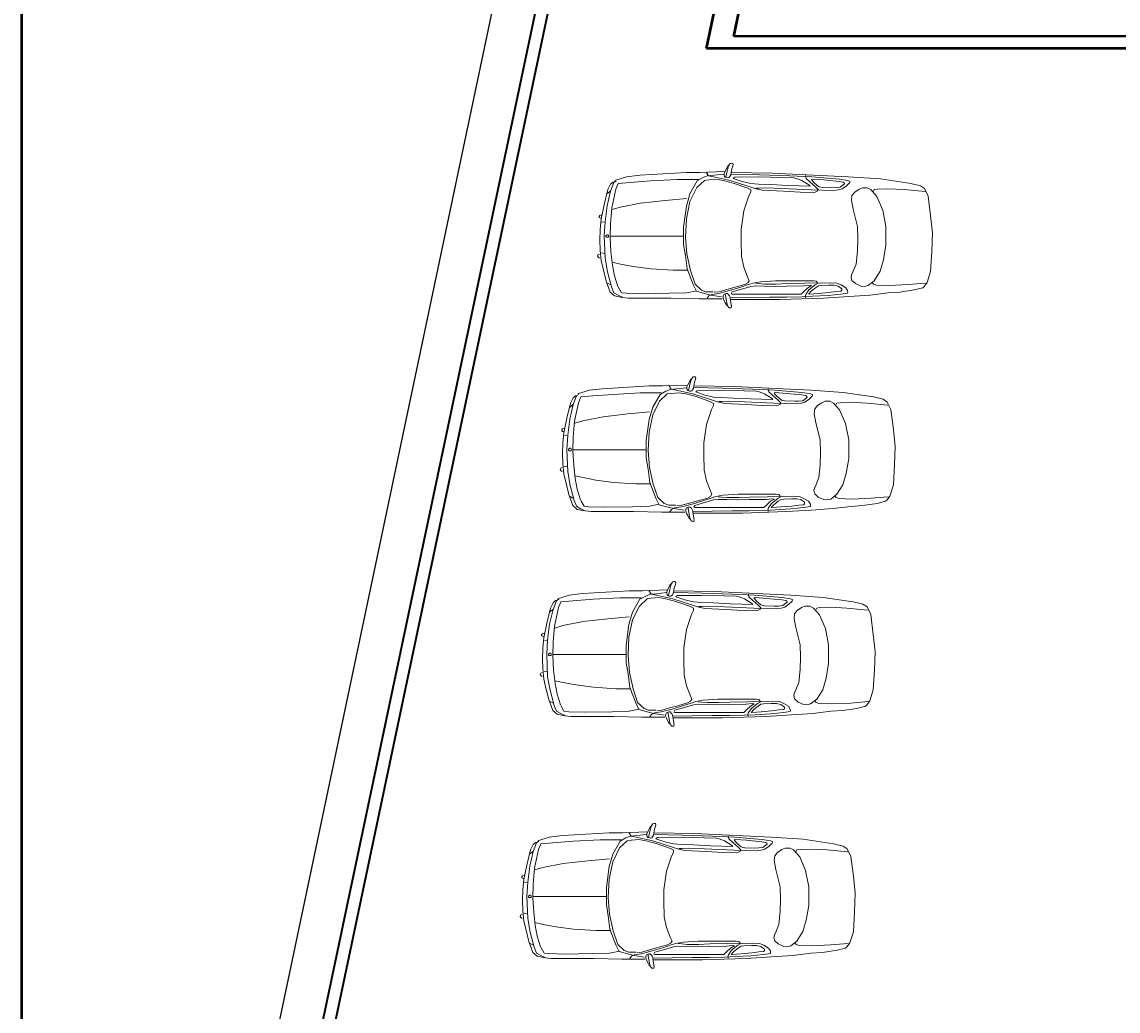
# Model space of a CAD drawing. Units: millimetres. Extents: x 2134 to 3363, y 1052 to 3233.
# Tile 2 of 11: x 2134 to 2539, y 1417 to 1782. Entities that reach past the tile are written whole.
import ezdxf

# ---------------------------------------------------------------- set-up
doc = ezdxf.new("R2010")
doc.units = ezdxf.units.MM
for name, color, linetype, lineweight in [('A-ANNO-DIMS', 2, 'Continuous', 18), ('A-ANNO-TTLB', 7, 'Continuous', 50), ('A-SITE-PRKG', 8, 'Continuous', 13), ('A-WALL', 7, 'Continuous', 50), ('C-PROP', 6, 'Continuous', 35)]:
    doc.layers.add(name, color=color, linetype=linetype, lineweight=lineweight)
doc.styles.get("Standard").update_dxf_attribs({"font": 'arial.ttf'})
doc.dimstyles.new('ISO-25', dxfattribs={"dimtxt": 2.5, "dimasz": 2.5, "dimexe": 1.25, "dimexo": 0.625, "dimtad": 1, "dimtxsty": 'Standard', "dimcen": 2.5, "dimadec": 0, "dimazin": 0, "dimtfac": 1, "dimtmove": 0, "dimatfit": 3, "dimfxl": 1, "dimarcsym": 0})

# ---------------------------------------------------------------- blocks, each defined once
blk = doc.blocks.new('A$C52303110')
for p, q in [((-0.168, 1.141), (-0.185, 1.111)), ((-0.162, 1.148), (-0.168, 1.141)), ((-0.142, 1.15), (-0.162, 1.148)), ((-0.13, 1.15), (-0.142, 1.15)), ((-0.123, 1.145), (-0.13, 1.15)), ((-0.117, 1.134), (-0.123, 1.145)), ((-0.123, 1.109), (-0.117, 1.134)), ((-1.693, 0.951), (-1.496, 0.973)), ((-1.496, 0.973), (-0.807, 1.016)), ((-0.807, 1.016), (-0.61, 1.016)), ((-0.61, 1.016), (-0.252, 1.027)), ((-0.517, 1.02), (-0.48, 0.966)), ((-0.256, 0.988), (-0.404, 0.972)), ((-0.237, 1.032), (-0.251, 1.001)), ((-0.251, 1.001), (-0.25, 0.98)), ((-0.25, 0.98), (-0.245, 0.957)), ((-0.198, 1.106), (-0.237, 1.032)), ((-0.206, 1.035), (-0.226, 0.944)), ((-0.185, 1.111), (-0.206, 1.035)), ((-0.184, 1.117), (-0.198, 1.106)), ((-0.167, 0.957), (-0.154, 0.98)), ((-0.154, 0.98), (-0.148, 1.013)), ((-0.148, 1.013), (-0.144, 1.04)), ((-0.145, 0.991), (0.272, 0.981)), ((-0.144, 1.04), (-0.137, 1.07)), ((-0.144, 1.016), (0.455, 1.005)), ((-0.137, 1.07), (-0.123, 1.109)), ((0.272, 0.981), (0.721, 0.966)), ((0.455, 1.005), (1.583, 0.951)), ((-1.969, 0.76), (-1.928, 0.839)), ((-1.928, 0.839), (-1.887, 0.875)), ((-1.928, 0.738), (-1.881, 0.868)), ((-1.881, 0.868), (-1.846, 0.889)), ((-1.863, 0.896), (-1.693, 0.951)), ((-1.852, 0.767), (-1.816, 0.853)), ((-1.816, 0.853), (-1.64, 0.868)), ((-1.64, 0.868), (-1.339, 0.889)), ((-1.339, 0.889), (-0.939, 0.911)), ((-0.939, 0.911), (-0.698, 0.911)), ((-0.647, 0.889), (-0.755, 0.7)), ((-0.698, 0.911), (-0.627, 0.911)), ((-0.539, 0.897), (-0.654, 0.79)), ((-0.56, 0.938), (-0.647, 0.889)), ((-0.499, 0.963), (-0.56, 0.938)), ((-0.479, 0.905), (-0.539, 0.897)), ((-0.404, 0.972), (-0.499, 0.963)), ((-0.48, 0.966), (-0.383, 0.946)), ((-0.371, 0.914), (-0.479, 0.905)), ((-0.383, 0.946), (-0.161, 0.897)), ((-0.263, 0.897), (-0.371, 0.914)), ((-0.115, 0.856), (-0.263, 0.897)), ((-0.245, 0.957), (-0.234, 0.947)), ((-0.234, 0.947), (-0.213, 0.938)), ((-0.213, 0.938), (-0.192, 0.936)), ((-0.192, 0.936), (-0.179, 0.942)), ((-0.179, 0.942), (-0.167, 0.957)), ((-0.161, 0.897), (0.098, 0.813)), ((-0.119, 0.926), (-0.109, 0.937)), ((0.017, 0.88), (-0.119, 0.926)), ((0.101, 0.782), (-0.115, 0.856)), ((-0.109, 0.937), (-0.091, 0.944)), ((-0.091, 0.944), (0.26, 0.948)), ((0.143, 0.85), (0.017, 0.88)), ((0.098, 0.813), (0.203, 0.778)), ((0.257, 0.843), (0.143, 0.85)), ((0.441, 0.835), (0.257, 0.843)), ((0.26, 0.948), (0.598, 0.941)), ((0.69, 0.824), (0.441, 0.835)), ((0.598, 0.941), (0.777, 0.937)), ((1.022, 0.813), (0.69, 0.824)), ((0.721, 0.966), (1.045, 0.951)), ((0.777, 0.937), (0.817, 0.926)), ((0.817, 0.926), (0.897, 0.896)), ((0.897, 0.896), (1.001, 0.832)), ((0.956, 0.951), (0.952, 0.971)), ((0.96, 0.926), (0.956, 0.951)), ((1.016, 0.877), (0.96, 0.926)), ((1.001, 0.832), (1.022, 0.813)), ((1.105, 0.798), (1.016, 0.877)), ((1.038, 0.912), (1.054, 0.916)), ((1.043, 0.899), (1.038, 0.912)), ((1.082, 0.858), (1.043, 0.899)), ((1.045, 0.951), (1.453, 0.917)), ((1.054, 0.916), (1.221, 0.903)), ((1.141, 0.807), (1.082, 0.858)), ((1.221, 0.903), (1.447, 0.882)), ((1.447, 0.882), (1.506, 0.871)), ((1.453, 0.917), (1.579, 0.897)), ((1.508, 0.83), (1.464, 0.796)), ((1.555, 0.818), (1.494, 0.773)), ((1.506, 0.871), (1.524, 0.86)), ((1.527, 0.847), (1.508, 0.83)), ((1.524, 0.86), (1.527, 0.847)), ((1.603, 0.862), (1.555, 0.818)), ((1.579, 0.897), (1.611, 0.882)), ((1.583, 0.951), (2.058, 0.918)), ((1.611, 0.882), (1.603, 0.862)), ((2.058, 0.918), (2.505, 0.852)), ((2.505, 0.852), (2.648, 0.819)), ((2.648, 0.819), (2.711, 0.776)), ((-2.022, 0.537), (-1.969, 0.76)), ((-1.981, 0.523), (-1.928, 0.738)), ((-1.975, 0.702), (-1.934, 0.738)), ((-1.91, 0.494), (-1.852, 0.767)), ((-0.755, 0.7), (-0.809, 0.518)), ((-0.654, 0.79), (-0.755, 0.585)), ((0.04, 0.445), (0.115, 0.667)), ((0.142, 0.757), (0.101, 0.782)), ((0.115, 0.667), (0.142, 0.724)), ((0.142, 0.724), (0.142, 0.757)), ((0.203, 0.778), (0.312, 0.754)), ((0.268, 0.783), (0.22, 0.783)), ((0.361, 0.788), (0.268, 0.783)), ((0.312, 0.754), (0.624, 0.739)), ((0.6, 0.778), (0.361, 0.788)), ((1.037, 0.759), (0.6, 0.778)), ((0.624, 0.739), (0.871, 0.724)), ((0.871, 0.724), (1.077, 0.719)), ((1.364, 0.748), (1.037, 0.759)), ((1.077, 0.719), (1.13, 0.739)), ((1.138, 0.763), (1.105, 0.798)), ((1.13, 0.739), (1.138, 0.763)), ((1.159, 0.801), (1.141, 0.807)), ((1.199, 0.794), (1.159, 0.801)), ((1.338, 0.788), (1.199, 0.794)), ((1.403, 0.79), (1.338, 0.788)), ((1.437, 0.759), (1.364, 0.748)), ((1.464, 0.796), (1.403, 0.79)), ((1.494, 0.773), (1.437, 0.759)), ((1.638, 0.675), (1.632, 0.604)), ((1.678, 0.724), (1.638, 0.675)), ((1.742, 0.767), (1.678, 0.724)), ((1.794, 0.788), (1.742, 0.767)), ((1.863, 0.788), (1.794, 0.788)), ((1.915, 0.76), (1.863, 0.788)), ((2.007, 0.661), (1.915, 0.76)), ((1.955, 0.738), (1.967, 0.76)), ((1.967, 0.76), (2.013, 0.767)), ((2.094, 0.457), (2.007, 0.661)), ((2.013, 0.767), (2.169, 0.774)), ((2.169, 0.774), (2.411, 0.76)), ((2.411, 0.76), (2.717, 0.731)), ((2.711, 0.776), (2.765, 0.666)), ((2.765, 0.666), (2.8, 0.371)), ((-2.069, 0.322), (-2.022, 0.537)), ((-2.01, 0.285), (-1.981, 0.523)), ((-1.928, 0.257), (-1.91, 0.494)), ((-1.904, 0.465), (-1.787, 0.501)), ((-1.787, 0.501), (-1.487, 0.559)), ((-1.487, 0.559), (-1.122, 0.602)), ((-1.122, 0.602), (-0.804, 0.631)), ((-0.809, 0.518), (-0.849, 0.206)), ((-0.755, 0.585), (-0.809, 0.329)), ((1.632, 0.604), (1.655, 0.471)), ((-2.087, 0.379), (-2.099, 0.364)), ((-2.099, 0.364), (-2.099, 0.35)), ((-2.099, 0.35), (-2.087, 0.343)), ((-2.064, 0.386), (-2.087, 0.379)), ((-2.087, 0.343), (-2.069, 0.336)), ((-0.809, 0.329), (-0.823, 0.058)), ((0, 0.173), (0.04, 0.445)), ((1.655, 0.471), (1.718, 0.217)), ((2.14, 0.217), (2.094, 0.457)), ((2.8, 0.371), (2.828, 0.12)), ((-2.087, 0.012), (-2.081, 0.17)), ((-2.081, 0.17), (-2.069, 0.322)), ((-2.057, 0.278), (-2.022, 0.285)), ((-2.022, 0.077), (-2.01, 0.285)), ((-1.934, 0.055), (-1.928, 0.257)), ((-0.849, 0.206), (-0.849, -0.049)), ((0, 0), (0, 0.173)), ((1.718, 0.217), (1.724, 0.033)), ((2.14, -0.058), (2.14, 0.217)), ((-2.081, -0.132), (-2.087, 0.012)), ((-2.01, -0.254), (-2.022, 0.077)), ((-1.981, 0.093), (-1.999, 0.079)), ((-1.999, 0.079), (-1.999, 0.064)), ((-1.999, 0.057), (-1.97, 0.057)), ((-1.963, 0.093), (-1.981, 0.093)), ((-1.97, 0.057), (-1.958, 0.057)), ((-1.958, 0.079), (-1.963, 0.093)), ((-1.958, 0.057), (-1.958, 0.079)), ((-1.922, -0.16), (-1.934, 0.055)), ((-1.926, 0.072), (-0.858, 0.072)), ((-0.823, 0.058), (-0.802, -0.19)), ((0.007, -0.23), (0, 0)), ((1.724, 0.033), (1.718, -0.15)), ((2.828, 0.12), (2.819, -0.153)), ((-2.069, -0.29), (-2.081, -0.132)), ((-1.898, -0.354), (-1.922, -0.16)), ((-0.849, -0.049), (-0.823, -0.214)), ((1.718, -0.15), (1.701, -0.34)), ((2.105, -0.277), (2.14, -0.058)), ((2.819, -0.153), (2.8, -0.448)), ((-2.11, -0.2), (-2.122, -0.221)), ((-2.122, -0.221), (-2.11, -0.236)), ((-2.093, -0.193), (-2.11, -0.2)), ((-2.11, -0.236), (-2.093, -0.25)), ((-2.04, -0.405), (-2.069, -0.29)), ((-2.064, -0.175), (-2.016, -0.182)), ((-1.975, -0.455), (-2.01, -0.254)), ((-1.903, -0.313), (-1.782, -0.341)), ((-0.823, -0.214), (-0.796, -0.412)), ((-0.802, -0.19), (-0.748, -0.436)), ((0.04, -0.387), (0.007, -0.23)), ((2.053, -0.446), (2.105, -0.277)), ((-1.993, -0.592), (-2.04, -0.405)), ((-1.916, -0.678), (-1.975, -0.455)), ((-1.869, -0.512), (-1.898, -0.354)), ((-1.782, -0.341), (-1.593, -0.376)), ((-1.593, -0.376), (-1.335, -0.411)), ((-1.335, -0.411), (-1.002, -0.432)), ((-1.002, -0.432), (-0.784, -0.432)), ((-0.796, -0.412), (-0.708, -0.642)), ((-0.748, -0.436), (-0.681, -0.634)), ((0.094, -0.527), (0.04, -0.387)), ((1.638, -0.481), (1.626, -0.531)), ((1.701, -0.34), (1.643, -0.481)), ((1.967, -0.587), (2.053, -0.446)), ((2.8, -0.448), (2.747, -0.612)), ((-1.934, -0.754), (-1.993, -0.592)), ((-1.975, -0.62), (-1.934, -0.642)), ((-1.822, -0.671), (-1.869, -0.512)), ((-0.708, -0.642), (-0.661, -0.741)), ((-0.681, -0.634), (-0.586, -0.724)), ((-0.088, -0.683), (0.054, -0.642)), ((-0.002, -0.68), (0.109, -0.643)), ((0.054, -0.642), (0.101, -0.617)), ((0.121, -0.585), (0.094, -0.527)), ((0.101, -0.617), (0.121, -0.585)), ((0.109, -0.643), (0.178, -0.62)), ((0.178, -0.62), (0.288, -0.601)), ((0.266, -0.629), (0.212, -0.624)), ((0.346, -0.634), (0.266, -0.629)), ((0.288, -0.601), (0.506, -0.587)), ((0.518, -0.634), (0.346, -0.634)), ((0.506, -0.587), (0.881, -0.587)), ((0.682, -0.629), (0.518, -0.634)), ((0.943, -0.624), (0.682, -0.629)), ((0.881, -0.587), (1.069, -0.587)), ((1.118, -0.615), (0.943, -0.624)), ((1.092, -0.648), (1, -0.722)), ((1.069, -0.587), (1.107, -0.592)), ((1.13, -0.629), (1.092, -0.648)), ((1.107, -0.592), (1.122, -0.606)), ((1.161, -0.62), (1.118, -0.615)), ((1.122, -0.606), (1.13, -0.629)), ((1.314, -0.615), (1.161, -0.62)), ((1.413, -0.62), (1.314, -0.615)), ((1.478, -0.648), (1.413, -0.62)), ((1.547, -0.69), (1.478, -0.648)), ((1.626, -0.531), (1.638, -0.58)), ((1.638, -0.58), (1.69, -0.629)), ((1.69, -0.629), (1.771, -0.664)), ((1.875, -0.657), (1.967, -0.587)), ((1.938, -0.615), (1.955, -0.636)), ((1.955, -0.636), (2.001, -0.65)), ((2.186, -0.657), (2.469, -0.643)), ((2.469, -0.643), (2.723, -0.622)), ((2.747, -0.612), (2.711, -0.667)), ((-1.872, -0.809), (-1.934, -0.754)), ((-1.881, -0.764), (-1.916, -0.678)), ((-1.816, -0.8), (-1.881, -0.764)), ((-1.755, -0.831), (-1.872, -0.809)), ((-1.816, -0.678), (-1.769, -0.764)), ((-1.752, -0.829), (-1.816, -0.8)), ((-1.769, -0.764), (-1.699, -0.771)), ((-1.699, -0.771), (-1.463, -0.778)), ((-1.463, -0.778), (-1.057, -0.771)), ((-1.057, -0.771), (-0.804, -0.764)), ((-0.804, -0.764), (-0.657, -0.735)), ((-0.661, -0.741), (-0.573, -0.766)), ((-0.586, -0.724), (-0.519, -0.749)), ((-0.573, -0.766), (-0.445, -0.799)), ((-0.519, -0.749), (-0.445, -0.749)), ((-0.477, -0.811), (-0.434, -0.788)), ((-0.445, -0.749), (-0.411, -0.749)), ((-0.445, -0.799), (-0.29, -0.823)), ((-0.434, -0.788), (-0.331, -0.774)), ((-0.398, -0.757), (-0.324, -0.749)), ((-0.331, -0.774), (-0.171, -0.732)), ((-0.324, -0.749), (-0.209, -0.716)), ((-0.267, -0.838), (-0.264, -0.809)), ((-0.264, -0.809), (-0.255, -0.789)), ((-0.255, -0.789), (-0.236, -0.778)), ((-0.236, -0.778), (-0.216, -0.773)), ((-0.232, -0.803), (-0.233, -0.779)), ((-0.221, -0.857), (-0.232, -0.803)), ((-0.216, -0.773), (-0.2, -0.775)), ((-0.209, -0.716), (-0.088, -0.683)), ((-0.2, -0.775), (-0.184, -0.792)), ((-0.184, -0.792), (-0.171, -0.809)), ((-0.171, -0.732), (-0.002, -0.68)), ((-0.171, -0.809), (-0.164, -0.829)), ((-0.132, -0.75), (-0.148, -0.778)), ((-0.148, -0.778), (-0.132, -0.783)), ((0.028, -0.704), (-0.132, -0.75)), ((-0.132, -0.783), (-0.067, -0.783)), ((-0.067, -0.783), (0.147, -0.783)), ((0.143, -0.671), (0.028, -0.704)), ((0.216, -0.662), (0.143, -0.671)), ((0.147, -0.783), (0.529, -0.783)), ((0.342, -0.666), (0.216, -0.662)), ((0.503, -0.671), (0.342, -0.666)), ((0.671, -0.666), (0.503, -0.671)), ((0.529, -0.783), (0.786, -0.783)), ((0.92, -0.662), (0.671, -0.666)), ((0.786, -0.783), (0.889, -0.783)), ((0.889, -0.783), (0.927, -0.746)), ((1.011, -0.652), (0.92, -0.662)), ((0.927, -0.746), (0.985, -0.69)), ((0.954, -0.788), (0.946, -0.82)), ((1, -0.722), (0.954, -0.788)), ((0.985, -0.69), (1.042, -0.657)), ((1.034, -0.741), (0.996, -0.783)), ((1.004, -0.783), (1.145, -0.774)), ((1.042, -0.657), (1.011, -0.652)), ((1.099, -0.69), (1.034, -0.741)), ((1.057, -0.816), (1.287, -0.802)), ((1.141, -0.662), (1.099, -0.69)), ((1.18, -0.657), (1.141, -0.662)), ((1.145, -0.774), (1.298, -0.76)), ((1.294, -0.652), (1.18, -0.657)), ((1.287, -0.802), (1.474, -0.783)), ((1.371, -0.652), (1.294, -0.652)), ((1.298, -0.76), (1.405, -0.746)), ((1.432, -0.666), (1.371, -0.652)), ((1.405, -0.746), (1.474, -0.741)), ((1.489, -0.704), (1.432, -0.666)), ((1.474, -0.741), (1.489, -0.727)), ((1.474, -0.783), (1.574, -0.769)), ((1.489, -0.727), (1.489, -0.704)), ((1.574, -0.732), (1.547, -0.69)), ((1.577, -0.76), (1.574, -0.732)), ((1.574, -0.769), (1.577, -0.76)), ((1.905, -0.798), (1.592, -0.82)), ((1.771, -0.664), (1.817, -0.671)), ((1.817, -0.671), (1.875, -0.657)), ((2.174, -0.766), (1.905, -0.798)), ((2.001, -0.65), (2.186, -0.657)), ((2.344, -0.754), (2.174, -0.766)), ((2.559, -0.722), (2.344, -0.754)), ((2.684, -0.689), (2.559, -0.722)), ((2.711, -0.667), (2.684, -0.689)), ((-1.666, -0.842), (-1.755, -0.831)), ((-1.55, -0.842), (-1.666, -0.842)), ((-1.039, -0.842), (-1.55, -0.842)), ((-0.619, -0.853), (-1.039, -0.842)), ((-0.279, -0.853), (-0.619, -0.853)), ((-0.503, -0.844), (-0.477, -0.811)), ((-0.254, -0.869), (-0.267, -0.838)), ((-0.233, -0.91), (-0.254, -0.869)), ((-0.217, -0.944), (-0.233, -0.91)), ((-0.205, -0.935), (-0.221, -0.857)), ((-0.2, -0.956), (-0.217, -0.944)), ((-0.196, -0.961), (-0.205, -0.935)), ((-0.192, -0.972), (-0.196, -0.961)), ((-0.164, -0.829), (-0.161, -0.849)), ((-0.161, -0.849), (-0.152, -0.906)), ((-0.155, -0.839), (0.124, -0.835)), ((-0.01, -0.864), (-0.153, -0.864)), ((-0.152, -0.906), (-0.143, -0.972)), ((0.572, -0.864), (-0.01, -0.864)), ((0.124, -0.835), (0.419, -0.83)), ((0.419, -0.83), (0.675, -0.83)), ((1.216, -0.842), (0.572, -0.864)), ((0.675, -0.83), (0.9, -0.825)), ((0.9, -0.825), (1.057, -0.816)), ((0.946, -0.82), (0.95, -0.839)), ((1.592, -0.82), (1.216, -0.842)), ((-0.178, -0.984), (-0.192, -0.972)), ((-0.166, -0.986), (-0.178, -0.984)), ((-0.152, -0.987), (-0.166, -0.986)), ((-0.146, -0.982), (-0.152, -0.987)), ((-0.143, -0.972), (-0.146, -0.982))]:
    blk.add_line(p, q)
blk = doc.blocks.new('*D8')
at = {"layer": 'A-ANNO-DIMS', "color": 0, "lineweight": -2, "transparency": 16777216}
for p, q in [((2457.75, 2425.14), (2441.71, 2428.51)), ((2442.41, 2425.81), (2184.54, 1200.99)), ((2198.85, 1195.42), (2182.8, 1198.8))]:
    blk.add_line(p, q, dxfattribs=at)
at = {"layer": 'A-ANNO-DIMS', "color": 0, "transparency": 16777216}
for points in [[(2442.01, 2425.9), (2442.82, 2425.72), (2442.93, 2428.26)], [(2184.14, 1201.07), (2184.95, 1200.9), (2184.03, 1198.54)]]:
    blk.add_solid(points, dxfattribs=at)
at = {"layer": 'Defpoints', "color": 0, "transparency": 16777216}
for p in [(2458.36, 2425.01), (2184.03, 1198.54), (2199.46, 1195.29)]:
    blk.add_point(p, dxfattribs=at)
at = {"layer": 'A-ANNO-DIMS', "color": 0, "transparency": 16777216, "insert": (2311.4, 1813.84), "char_height": 2.5, "attachment_point": 5, "rotation": 78.1108}
blk.add_mtext('1256,67', dxfattribs=at)
blk = doc.blocks.new('*D10')
at = {"layer": 'A-ANNO-DIMS', "color": 0, "lineweight": -2, "transparency": 16777216}
for p, q in [((3164.66, 1769.83), (3180.9, 1742.8)), ((3178.12, 1742.58), (2221.66, 1167.89)), ((2203.92, 1192.56), (2220.16, 1165.53))]:
    blk.add_line(p, q, dxfattribs=at)
at = {"layer": 'A-ANNO-DIMS', "color": 0, "transparency": 16777216}
for points in [[(3177.9, 1742.94), (3178.33, 1742.23), (3180.26, 1743.87)], [(2221.44, 1168.24), (2221.87, 1167.53), (2219.52, 1166.6)]]:
    blk.add_solid(points, dxfattribs=at)
at = {"layer": 'Defpoints', "color": 0, "transparency": 16777216}
for p in [(3164.34, 1770.37), (2203.6, 1193.09), (2219.52, 1166.6)]:
    blk.add_point(p, dxfattribs=at)
at = {"layer": 'A-ANNO-DIMS', "color": 0, "transparency": 16777216, "insert": (2674.71, 1442.59), "char_height": 2.5, "attachment_point": 5, "rotation": 31}
blk.add_mtext('1120,83', dxfattribs=at)
blk = doc.blocks.new('*D6')
at = {"layer": 'A-ANNO-DIMS', "color": 0, "lineweight": -2, "transparency": 16777216}
blk.add_arc((2458.36, 2425.01), 20.29, 94.064, 251.0467, dxfattribs=at)
at = {"layer": 'A-ANNO-DIMS', "color": 0, "transparency": 16777216}
for points in [[(2456.92, 2445.66), (2456.93, 2444.83), (2459.42, 2445.27)], [(2451.88, 2406.22), (2451.66, 2405.42), (2454.18, 2405.15)]]:
    blk.add_solid(points, dxfattribs=at)
at = {"layer": 'Defpoints', "color": 0, "transparency": 16777216}
for p in [(2491.84, 3063.82), (2441.94, 2436.92), (2458.36, 2425.01), (2458.36, 2425.01), (2197.07, 1183.92)]:
    blk.add_point(p, dxfattribs=at)
at = {"layer": 'A-ANNO-DIMS', "color": 0, "transparency": 16777216, "insert": (2436.38, 2427.88), "char_height": 2.5, "attachment_point": 5, "rotation": 82.5554}
blk.add_mtext('171°', dxfattribs=at)

msp = doc.modelspace()

# ---------------------------------------------------------------- linework, layer by layer
at = {"layer": 'A-ANNO-TTLB', "ltscale": 0.5}
msp.add_lwpolyline([(2134.34, 3233.23), (3362.77, 3233.23), (3362.77, 1152.237), (2134.34, 1152.237)], close=True, dxfattribs=at)
at = {"layer": 'A-WALL'}
for p, q in [((2386.865, 1772.344), (2522.51, 2416.625)), ((2396.963, 1776.846), (2531.497, 2416.154)), ((2396.964, 1772.346), (2386.865, 1772.344))]:
    msp.add_line(p, q, dxfattribs=at)
for points in [[(2754.719, 1776.895), (2650.315, 1776.895), (2396.963, 1776.846)], [(2754.719, 1772.395), (2650.315, 1772.395), (2396.964, 1772.346)]]:
    msp.add_lwpolyline(points, dxfattribs=at)
at = {"layer": 'C-PROP'}
for p, q in [((2197.066, 1183.92), (2458.361, 2425.007)), ((2203.596, 1193.093), (2462.764, 2424.08))]:
    msp.add_line(p, q, dxfattribs=at)

# ---------------------------------------------------------------- block references
at = {"layer": 'A-SITE-PRKG', "xscale": 24.97117926718032, "yscale": 24.97117926718032, "zscale": 24.97117926718032}
for p in [(2399.634, 1701.337), (2385.875, 1622.56), (2378.47, 1546.952), (2371.122, 1457.677)]:
    msp.add_blockref('A$C52303110', p, dxfattribs=at)

# ---------------------------------------------------------------- dimensions: what is measured, and where the dimension line sits
at = {"layer": 'A-ANNO-DIMS'}
dim = msp.add_angular_dim_2l(base=(2441.938, 2436.923), line1=((2197.066, 1183.92), (2458.361, 2425.007)), line2=((2458.361, 2425.007), (2491.839, 3063.82)), dimstyle='ISO-25', override={"dimclrd": 0, "dimclre": 0, "dimclrt": 0}, dxfattribs=at)
dim.commit()
dim.dimension.update_dxf_attribs({"geometry": '*D6', "text_midpoint": (2436.377, 2427.88)})
dim = msp.add_aligned_dim(p1=(2458.361, 2425.007), p2=(2199.46, 1195.291), distance=-15.77, dimstyle='ISO-25', override={"dimclrd": 0, "dimclre": 0, "dimclrt": 0}, dxfattribs=at)
dim.commit()
dim.dimension.update_dxf_attribs({"geometry": '*D8', "text_midpoint": (2311.397, 1813.836)})
dim = msp.add_linear_dim(base=(2219.5153, 1166.599), p1=(3164.339, 1770.3661), p2=(2203.5959, 1193.0934), angle=211, dimstyle='ISO-25', override={"dimclrd": 0, "dimclre": 0, "dimclrt": 0}, dxfattribs=at)
dim.commit()
dim.dimension.update_dxf_attribs({"geometry": '*D10', "text_midpoint": (2675.8085, 1440.7677), "dimtype": 161})

doc.saveas('drawing.dxf')
